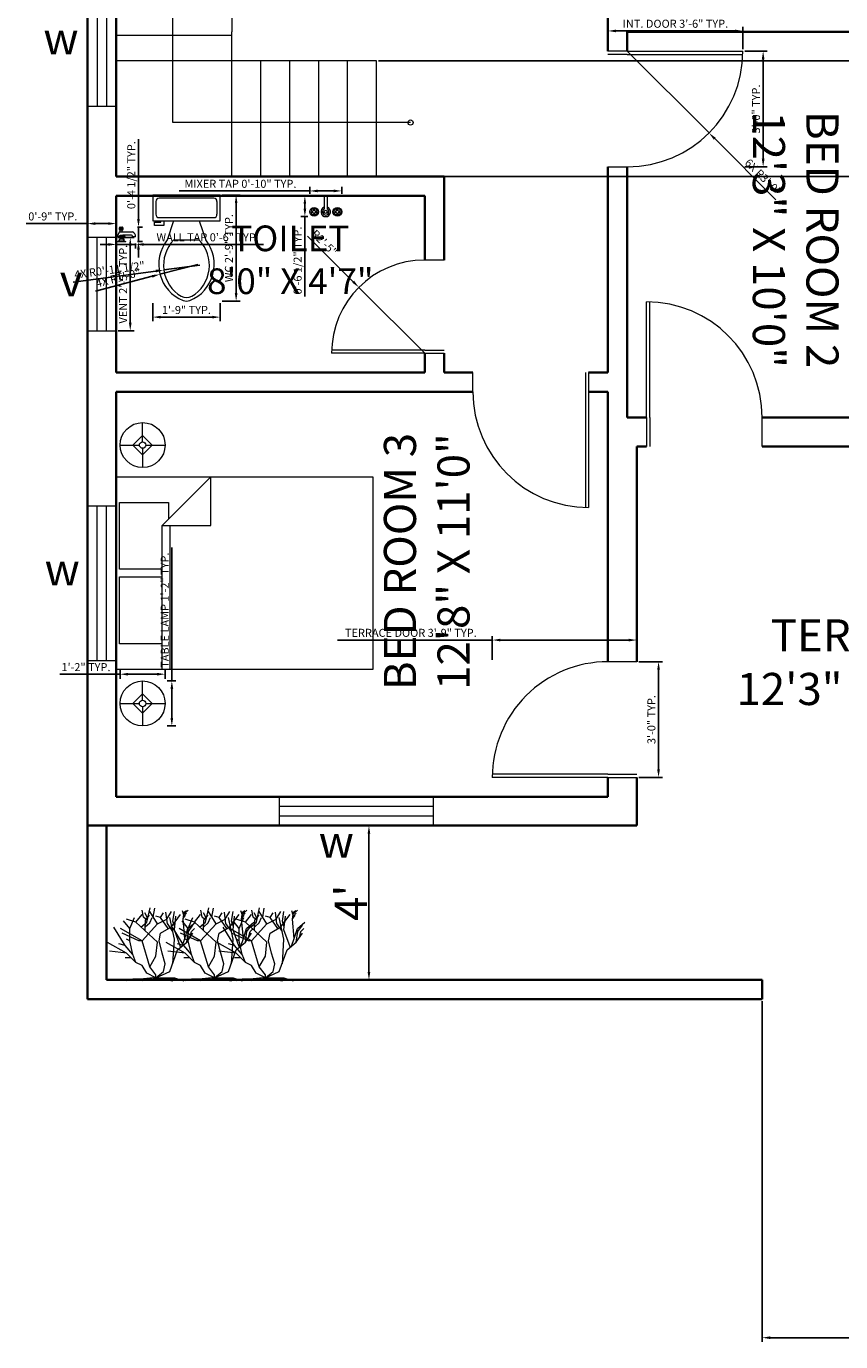
# Model space of a CAD drawing. Units: inches. Extents: x 2729 to 3178, y 5006 to 5809.
# Tile 1 of 4: x 2729 to 2983, y 5006 to 5415. Entities that reach past the tile are written whole.
import ezdxf

# ---------------------------------------------------------------- set-up
doc = ezdxf.new("R2010")
doc.units = ezdxf.units.IN
doc.layers.get('Defpoints').update_dxf_attribs({"color": 72})
for name, color, linetype, lineweight in [('A-ANNO-DIMS', 2, 'Continuous', 18), ('A-ANNO-TEXT', 7, 'Continuous', 18), ('A-AREA-IDEN', 7, 'Continuous', 25), ('A-DOOR', 4, 'Continuous', 18), ('A-FLOR-FIXT', 9, 'Continuous', 18), ('A-FLOR-STRS', 7, 'Continuous', 18), ('A-FURN', 8, 'Continuous', 18), ('A-GLAZ', 4, 'Continuous', 18), ('A-WALL', 7, 'Continuous', 35), ('L-PLNT', 72, 'Continuous', 13)]:
    doc.layers.add(name, color=color, linetype=linetype, lineweight=lineweight)
doc.styles.get("Standard").update_dxf_attribs({"font": 'arial.ttf'})
doc.dimstyles.new('ISO-25', dxfattribs={"dimtxt": 2.5, "dimasz": 2.5, "dimexe": 1.25, "dimexo": 0.625, "dimtad": 1, "dimdec": 0, "dimlunit": 3, "dimtxsty": 'Standard', "dimcen": 2.5, "dimadec": 0, "dimazin": 0, "dimtfac": 1, "dimtdec": 0, "dimtmove": 0, "dimatfit": 3, "dimfxl": 1, "dimarcsym": 0})

# ---------------------------------------------------------------- blocks, each defined once
blk = doc.blocks.new('Toilet - top')
for p, q in [((9.5, -6), (9.5, -2)), ((-8, -8.5), (-8, -8)), ((-7, -8), (-7, -9.5)), ((-4, -8), (-6, -14)), ((4, -8), (6, -14)), ((-10, -8.5), (-8, -8.5)), ((-10, -9.5), (-10, -8.5)), ((-7, -9.5), (-10, -9.5)), ((4, -14), (-4, -14))]:
    blk.add_line(p, q)
blk.add_lwpolyline([(10.5, -8), (10.5, 0), (-10.5, 0), (-10.5, -8)], close=True)
for points in [[(-9.5, -2), (-9.5, -6)], [(8.5, -1), (-8.5, -1)], [(-8.5, -7), (8.5, -7)]]:
    blk.add_lwpolyline(points)
for centre, radius, start, end in [((-8.62, -1.88), 0.884, 81.8699, 188.1301), ((8.62, -1.88), 0.884, 351.8699, 98.1301), ((-8.62, -6.12), 0.884, 171.8699, 278.1301), ((8.62, -6.12), 0.884, 261.8699, 8.1301), ((3.52, -21.58), 12.17, 141.4691, 247.9714), ((4.2, -21.82), 11.33, 136.3677, 238.9468), ((-3.52, -21.58), 12.17, 292.0284, 38.5307), ((-4.2, -21.82), 11.33, 301.053, 43.6321), ((0, -27.88), 4, 245.7318, 294.2682), ((0, -29), 4, 254.8605, 285.1395)]:
    blk.add_arc(centre, radius, start, end)
blk = doc.blocks.new('Bed - Queen')
for p, q in [((0, -80.00003), (0, 0)), ((0, 0), (59.99999, 0)), ((59.99999, 0), (59.99999, -80.00003)), ((7.99999, -1.2), (28.79998, -1.2)), ((7.99999, -14.4), (7.99999, -1.2)), ((28.79998, -1.2), (28.79998, -14.4)), ((31.19999, -1.2), (51.99999, -1.2)), ((31.19999, -14.4), (31.19999, -1.2)), ((51.99999, -1.2), (51.99999, -16.4)), ((0, -14.4), (44.8, -14.4)), ((59.99999, -29.6), (44.8, -14.4)), ((44.8, -14.4), (44.8, -29.6)), ((44.8, -16.8), (0, -16.8)), ((51.99999, -16.4), (46.79936, -16.4)), ((44.8, -29.6), (59.99999, -29.6)), ((59.99999, -80.00003), (0, -80.00003))]:
    blk.add_line(p, q)
blk = doc.blocks.new('Lamp - Table')
for p, q in [((0, 7), (0, 1)), ((-1, 0), (-7, 0)), ((0, 3), (-3, 0)), ((-3, 0), (0, -3)), ((3, 0), (0, 3)), ((0, -3), (3, 0)), ((1, 0), (7, 0)), ((0, -1), (0, -7))]:
    blk.add_line(p, q)
for radius in [7, 1]:
    blk.add_circle((0, 0), radius)
blk = doc.blocks.new('Faucet - Bathroom top')
for p, q in [((-4.107, 0.125), (-4.375, 0.125)), ((-3.75, 0.4788), (-3.75, 0.75)), ((-3.5, 0.482), (-3.5, 0.75)), ((-3.1461, 0.125), (-2.875, 0.125)), ((3.143, 0.125), (2.875, 0.125)), ((3.5, 0.4788), (3.5, 0.75)), ((3.75, 0.482), (3.75, 0.75)), ((4.1039, 0.125), (4.375, 0.125)), ((-4.1039, -0.125), (-4.375, -0.125)), ((-3.75, -0.4821), (-3.75, -0.75)), ((-3.5, -0.4789), (-3.5, -0.75)), ((-3.143, -0.125), (-2.875, -0.125)), ((-0.5, -0.8639), (-0.5, -4.5)), ((0.5, -4.5), (0.5, -0.8631)), ((3.1461, -0.125), (2.875, -0.125)), ((3.5, -0.4821), (3.5, -0.75)), ((3.75, -0.4789), (3.75, -0.75)), ((4.107, -0.125), (4.375, -0.125))]:
    blk.add_line(p, q)
for centre, radius in [((-3.625, 0), 1.375), ((-4.625, 0), 0.2795), ((-3.625, 0), 0.5), ((-3.625, 1), 0.2795), ((-2.625, 0), 0.2795), ((0, 0), 0.5), ((3.625, 0), 1.375), ((2.625, 0), 0.2795), ((3.625, 0), 0.5), ((3.625, 1), 0.2795), ((4.625, 0), 0.2795), ((-3.625, -1), 0.2795), ((3.625, -1), 0.2795)]:
    blk.add_circle(centre, radius)
for centre, radius, start, end in [((-3.625, 0), 1, 105.2407, 164.2093), ((-3.625, 0), 1, 16.44125, 74.07887), ((0, 0), 1.5, 289.6514, 250.3603), ((0, 0), 1, 300.3431, 239.7554), ((3.625, 0), 1, 106.12, 164.0884), ((3.625, 0), 1, 16.23422, 73.90469), ((-3.625, 0), 1, 196.2342, 253.9047), ((-3.625, 0), 1, 286.12, 344.0884), ((3.625, 0), 1, 196.4413, 254.0789), ((3.625, 0), 1, 285.2407, 344.2093), ((0, -4.5), 0.5, 180, 0)]:
    blk.add_arc(centre, radius, start, end)
blk = doc.blocks.new('Faucet - Bathroom side')
for p, q in [((-0.625, 4.25), (0.375, 4.25)), ((-1.625, 0), (-1.375, 0)), ((-1.375, 0), (1.375, 0)), ((-0.88366, 0.25), (0.88424, 0.25)), ((0.375, 3.75), (-0.625, 3.75)), ((-0.625, 3), (3.375, 3)), ((-0.375, 1.625), (-0.625, 1.625)), ((-0.375, 1.375), (-0.625, 1.375)), ((0.48078, 0.75), (-0.47286, 0.75)), ((-0.375, 3), (-0.375, 3.5)), ((0.125, 3.5), (0.125, 3)), ((2.875, 2), (0.375, 2)), ((0.375, 1.625), (0.625, 1.625)), ((0.375, 1.375), (0.625, 1.375)), ((4.375, 1.5), (3.375, 1.5))]:
    blk.add_line(p, q)
for points in [[(-0.625, 3.75), (-0.625, 4.25)], [(-0.375, 4.5), (0.125, 4.5)], [(0.375, 4.25), (0.375, 3.75)], [(0.125, 3.5), (-0.375, 3.5)]]:
    blk.add_lwpolyline(points)
blk.add_lwpolyline([(-0.375, 1), (-0.375, 2), (0.375, 2), (0.375, 1)], close=True)
for centre in [(-0.875, 1.5), (0, 1.5), (0.875, 1.5)]:
    blk.add_circle(centre, 0.27951)
for centre, radius, start, end in [((-0.38253, 4.2575), 0.24259, 88.22243, 181.7776), ((0.13252, 4.2575), 0.24259, 358.2224, 91.77757), ((3.45929, -0.0281), 5.08436, 143.4467, 179.6834), ((-1.75, 1.375), 1.42522, 285.2551, 344.7449), ((-0.38253, 3.7424), 0.24259, 178.2224, 271.7776), ((0.13252, 3.7424), 0.24259, 268.2224, 1.777565), ((1.75, 1.375), 1.42522, 195.2551, 254.7449), ((-2.49562, -0.286), 3.38273, 9.709485, 29.48735), ((2.96867, 1.5936), 0.41699, 347.0192, 102.9808), ((2.70708, 1.4714), 1.66816, 0.9827695, 66.39737)]:
    blk.add_arc(centre, radius, start, end)
blk = doc.blocks.new('*U13')
for p, q in [((-377.952, 463.296), (-329.184, 524.256)), ((-316.7634, 502.285), (-327.6092, 559.9176)), ((-286.512, 498.3226), (-307.4416, 538.0736)), ((-290.3982, 464.5406), (-265.6078, 577.8246)), ((-207.264, 451.104), (-268.224, 548.64)), ((-240.792, 502.285), (-228.3968, 573.8368)), ((-182.88, 499.872), (-158.496, 536.448)), ((-129.1844, 450.6214), (-140.0302, 542.036)), ((-134.112, 487.68), (-97.536, 548.64)), ((-97.536, 426.72), (-24.384, 524.256)), ((-85.7758, 472.4908), (-73.3552, 548.005)), ((-12.9032, 555.9552), (-2.0574, 522.1732)), ((-5.1562, 486.3846), (2.5908, 542.036)), ((-0.508, 508.254), (22.7584, 536.067)), ((1.0414, 526.1356), (35.1536, 559.9176)), ((2.5908, 542.036), (21.209, 555.9552)), ((-463.296, 280.416), (-552.577, 423.037)), ((-426.72, 414.528), (-475.488, 475.488)), ((-377.952, 463.296), (-451.104, 487.68)), ((-426.72, 414.528), (-390.144, 499.872)), ((-207.264, 304.8), (-377.952, 463.296)), ((-338.455, 424.7896), (-290.3982, 464.5406)), ((-329.184, 316.992), (-207.264, 451.104)), ((-296.5958, 484.4034), (-316.7634, 502.285)), ((-305.8922, 396.9512), (-302.7934, 478.4344)), ((-304.3428, 426.7708), (-268.7066, 458.5716)), ((-302.7934, 478.4344), (-270.256, 518.1854)), ((-268.7066, 458.5716), (-250.0884, 500.3038)), ((-182.88, 499.872), (-219.456, 512.064)), ((-207.264, 451.104), (-134.112, 487.68)), ((-121.92, 414.528), (-182.88, 499.872)), ((-182.88, 377.952), (-97.536, 426.72)), ((-85.7758, 389.001), (-129.1844, 452.6026)), ((-73.152, 329.184), (-109.728, 499.872)), ((-70.2564, 426.7708), (-85.7758, 472.4908)), ((-73.152, 402.336), (-60.96, 512.064)), ((8.7884, 335.3562), (-5.1562, 486.3846)), ((-3.6068, 492.3536), (14.986, 518.1854)), ((33.6042, 412.8516), (92.5068, 464.5406)), ((36.576, 390.144), (73.152, 438.912)), ((-329.184, 316.992), (-499.872, 414.528)), ((-353.568, 316.992), (-487.68, 377.952)), ((-426.72, 316.992), (-451.104, 329.184)), ((-426.72, 316.992), (-426.72, 414.528)), ((-402.336, 207.264), (-426.72, 316.992)), ((-329.184, 316.992), (-353.568, 316.992)), ((-268.224, 109.728), (-329.184, 316.992)), ((-195.072, 316.992), (-182.88, 377.952)), ((-170.688, 219.456), (-195.072, 316.992)), ((-85.344, 134.112), (-73.152, 329.184)), ((-24.384, 268.224), (-73.152, 402.336)), ((-12.192, 274.32), (8.7884, 335.3562)), ((8.7884, 335.3562), (33.6042, 412.8516)), ((24.384, 304.8), (36.576, 390.144)), ((24.384, 304.8), (73.152, 377.952)), ((48.768, 341.376), (60.96, 390.144)), ((60.96, 390.144), (85.344, 414.528)), ((-451.104, 219.456), (-601.0402, 303.8094)), ((-451.104, 219.456), (-587.4512, 234.2388)), ((-463.296, 280.416), (-512.064, 292.608)), ((-402.336, 207.264), (-463.296, 280.416)), ((-377.952, 146.304), (-451.104, 219.456)), ((-219.456, 195.072), (-207.264, 304.8)), ((-146.304, 134.112), (-170.688, 219.456)), ((-109.728, 73.152), (-48.768, 243.84)), ((-48.768, 243.84), (24.384, 304.8)), ((-414.528, 182.88), (-463.296, 182.88)), ((-377.952, 146.304), (-402.336, 207.264)), ((-329.184, 121.92), (-377.952, 146.304)), ((-292.608, 60.96), (-329.184, 121.92)), ((-268.224, 109.728), (-219.456, 195.072)), ((-219.456, 48.768), (-268.224, 109.728)), ((-158.496, 73.152), (-146.304, 134.112)), ((-402.336, 12.192), (-451.104, 0)), ((-341.376, 12.192), (-402.336, 12.192)), ((-243.84, 24.384), (-341.376, 12.192)), ((-243.84, 24.384), (-329.184, 0)), ((-219.456, 24.384), (-292.608, 60.96)), ((-243.84, 24.384), (-195.072, 24.384)), ((-219.456, 24.384), (-109.728, 73.152)), ((-219.456, 24.384), (-158.496, 73.152)), ((-219.456, 24.384), (-219.456, 48.768)), ((-219.456, 24.384), (-73.152, 24.384)), ((-195.072, 24.384), (-158.496, 12.192)), ((-158.496, 12.192), (-85.344, 0)), ((-73.152, 24.384), (0, 0))]:
    blk.add_line(p, q)
blk = doc.blocks.new('*D17')
at = {"layer": 'A-ANNO-DIMS', "color": 0, "lineweight": -2, "transparency": 16777216}
for p, q in [((2754.8, 5166.64), (2837.06, 5166.64)), ((2835.81, 5164.14), (2835.81, 5121.14)), ((2754.8, 5118.64), (2837.06, 5118.64))]:
    blk.add_line(p, q, dxfattribs=at)
at = {"layer": 'A-ANNO-DIMS', "color": 0, "transparency": 16777216}
for points in [[(2835.39, 5164.14), (2836.23, 5164.14), (2835.81, 5166.64)], [(2835.39, 5121.14), (2836.23, 5121.14), (2835.81, 5118.64)]]:
    blk.add_solid(points, dxfattribs=at)
at = {"layer": 'Defpoints', "color": 0, "transparency": 16777216}
for p in [(2754.18, 5166.64), (2754.18, 5118.64), (2835.81, 5118.64)]:
    blk.add_point(p, dxfattribs=at)
at = {"layer": 'A-ANNO-DIMS', "color": 0, "transparency": 16777216, "insert": (2830.19, 5142.64), "char_height": 2.5, "attachment_point": 5, "rotation": 90}
blk.add_mtext("{\\H4x;4'}", dxfattribs=at)
blk = doc.blocks.new('WIN-48IN')
for p, q in [((48, 9), (0, 9)), ((0, 9), (0, 0)), ((48, 0), (48, 9)), ((48, 6), (0, 6)), ((0, 3), (48, 3)), ((0, 0), (48, 0))]:
    blk.add_line(p, q)
blk = doc.blocks.new('DOOR-36IN-JAMB6')
for p, q in [((0, 6), (0, 42)), ((1, 6), (1, 42)), ((0, 6), (0, 0)), ((1, 6), (1, 0)), ((36, 0), (36, 6))]:
    blk.add_line(p, q)
blk.add_arc((0, 6), 36, 0, 90)
blk = doc.blocks.new('VENT-29IN')
for p, q in [((29, 9), (0, 9)), ((0, 9), (0, 0)), ((29, 0), (29, 9)), ((29, 6), (0, 6)), ((0, 3), (29, 3)), ((0, 0), (29, 0))]:
    blk.add_line(p, q)
blk = doc.blocks.new('DOOR-36IN-JAMB9')
for p, q in [((0, 9), (0, 45)), ((1, 9), (1, 45)), ((0, 9), (0, 0)), ((1, 9), (1, 0)), ((36, 0), (36, 9))]:
    blk.add_line(p, q)
blk.add_arc((0, 9), 36, 0, 90)
blk = doc.blocks.new('*D29')
at = {"layer": 'A-ANNO-DIMS', "color": 0, "lineweight": -2, "transparency": 16777216}
for p, q in [((2774.48, 5211.66), (2774.48, 5253.23)), ((2773, 5211.66), (2775.73, 5211.66)), ((2774.48, 5200.16), (2774.48, 5209.16)), ((2773, 5197.66), (2775.73, 5197.66))]:
    blk.add_line(p, q, dxfattribs=at)
at = {"layer": 'A-ANNO-DIMS', "color": 0, "transparency": 16777216}
for points in [[(2774.06, 5209.16), (2774.9, 5209.16), (2774.48, 5211.66)], [(2774.06, 5200.16), (2774.9, 5200.16), (2774.48, 5197.66)]]:
    blk.add_solid(points, dxfattribs=at)
at = {"layer": 'Defpoints', "color": 0, "transparency": 16777216}
for p in [(2772.38, 5211.66), (2774.48, 5211.66), (2772.38, 5197.66)]:
    blk.add_point(p, dxfattribs=at)
at = {"layer": 'A-ANNO-DIMS', "color": 0, "transparency": 16777216, "insert": (2772.6, 5233.69), "char_height": 2.5, "attachment_point": 5, "rotation": 90}
blk.add_mtext('TABLE LAMP 1\'-2" TYP.', dxfattribs=at)
blk = doc.blocks.new('*D30')
at = {"layer": 'A-ANNO-DIMS', "color": 0, "lineweight": -2, "transparency": 16777216}
for p, q in [((2758.38, 5212.29), (2758.38, 5215.01)), ((2772.38, 5212.29), (2772.38, 5215.01)), ((2758.38, 5213.76), (2739.62, 5213.76)), ((2769.88, 5213.76), (2760.88, 5213.76))]:
    blk.add_line(p, q, dxfattribs=at)
at = {"layer": 'A-ANNO-DIMS', "color": 0, "transparency": 16777216}
for points in [[(2760.88, 5214.18), (2760.88, 5213.34), (2758.38, 5213.76)], [(2769.88, 5214.18), (2769.88, 5213.34), (2772.38, 5213.76)]]:
    blk.add_solid(points, dxfattribs=at)
at = {"layer": 'Defpoints', "color": 0, "transparency": 16777216}
for p in [(2758.38, 5213.76), (2758.38, 5211.66), (2772.38, 5211.66)]:
    blk.add_point(p, dxfattribs=at)
at = {"layer": 'A-ANNO-DIMS', "color": 0, "transparency": 16777216, "insert": (2747.75, 5215.64), "char_height": 2.5, "attachment_point": 5}
blk.add_mtext('1\'-2" TYP.', dxfattribs=at)
blk = doc.blocks.new('*D33')
at = {"layer": 'A-ANNO-DIMS', "color": 0, "lineweight": -2, "transparency": 16777216}
for p, q in [((2754.7, 5347.5), (2752.2, 5347.5)), ((2757.2, 5347.78), (2757.2, 5346.25)), ((2757.2, 5347.5), (2763.2, 5347.5)), ((2763.2, 5347.78), (2763.2, 5346.25)), ((2765.7, 5347.5), (2803.03, 5347.5))]:
    blk.add_line(p, q, dxfattribs=at)
at = {"layer": 'A-ANNO-DIMS', "color": 0, "transparency": 16777216}
for points in [[(2754.7, 5347.92), (2754.7, 5347.08), (2757.2, 5347.5)], [(2765.7, 5347.92), (2765.7, 5347.08), (2763.2, 5347.5)]]:
    blk.add_solid(points, dxfattribs=at)
at = {"layer": 'Defpoints', "color": 0, "transparency": 16777216}
for p in [(2757.2, 5348.4), (2763.2, 5348.4), (2763.2, 5347.5)]:
    blk.add_point(p, dxfattribs=at)
at = {"layer": 'A-ANNO-DIMS', "color": 0, "transparency": 16777216, "insert": (2785.61, 5349.4), "char_height": 2.5, "attachment_point": 5}
blk.add_mtext('WALL TAP 0\'-6" TYP.', dxfattribs=at)
blk = doc.blocks.new('*D34')
at = {"layer": 'A-ANNO-DIMS', "color": 0, "lineweight": -2, "transparency": 16777216}
for p, q in [((2764.1, 5355.4), (2764.1, 5380.22)), ((2763.82, 5352.9), (2765.35, 5352.9)), ((2764.1, 5348.4), (2764.1, 5352.9)), ((2763.82, 5348.4), (2765.35, 5348.4)), ((2764.1, 5345.9), (2764.1, 5343.4))]:
    blk.add_line(p, q, dxfattribs=at)
at = {"layer": 'A-ANNO-DIMS', "color": 0, "transparency": 16777216}
for points in [[(2763.68, 5355.4), (2764.51, 5355.4), (2764.1, 5352.9)], [(2763.68, 5345.9), (2764.51, 5345.9), (2764.1, 5348.4)]]:
    blk.add_solid(points, dxfattribs=at)
at = {"layer": 'Defpoints', "color": 0, "transparency": 16777216}
for p in [(2763.2, 5352.9), (2764.1, 5352.9), (2763.2, 5348.4)]:
    blk.add_point(p, dxfattribs=at)
at = {"layer": 'A-ANNO-DIMS', "color": 0, "transparency": 16777216, "insert": (2762.18, 5369.06), "char_height": 2.5, "attachment_point": 5, "rotation": 90}
blk.add_mtext('0\'-4 1/2" TYP.', dxfattribs=at)
blk = doc.blocks.new('*D35')
at = {"layer": 'A-ANNO-DIMS', "color": 0, "lineweight": -2, "transparency": 16777216}
for p, q in [((2910.18, 5408.26), (2910.18, 5415.19)), ((2912.68, 5413.94), (2949.68, 5413.94)), ((2952.18, 5408.26), (2952.18, 5415.19))]:
    blk.add_line(p, q, dxfattribs=at)
at = {"layer": 'A-ANNO-DIMS', "color": 0, "transparency": 16777216}
for points in [[(2912.68, 5414.35), (2912.68, 5413.52), (2910.18, 5413.94)], [(2949.68, 5414.35), (2949.68, 5413.52), (2952.18, 5413.94)]]:
    blk.add_solid(points, dxfattribs=at)
at = {"layer": 'Defpoints', "color": 0, "transparency": 16777216}
for p in [(2952.18, 5413.94), (2910.18, 5407.64), (2952.18, 5407.64)]:
    blk.add_point(p, dxfattribs=at)
at = {"layer": 'A-ANNO-DIMS', "color": 0, "transparency": 16777216, "insert": (2931.18, 5415.86), "char_height": 2.5, "attachment_point": 5}
blk.add_mtext('INT. DOOR 3\'-6" TYP.', dxfattribs=at)
blk = doc.blocks.new('*D36')
at = {"layer": 'A-ANNO-DIMS', "color": 0, "lineweight": -2, "transparency": 16777216}
for p, q in [((2952.8, 5407.64), (2959.73, 5407.64)), ((2958.48, 5405.14), (2958.48, 5374.14)), ((2952.8, 5371.64), (2959.73, 5371.64))]:
    blk.add_line(p, q, dxfattribs=at)
at = {"layer": 'A-ANNO-DIMS', "color": 0, "transparency": 16777216}
for points in [[(2958.06, 5405.14), (2958.9, 5405.14), (2958.48, 5407.64)], [(2958.06, 5374.14), (2958.9, 5374.14), (2958.48, 5371.64)]]:
    blk.add_solid(points, dxfattribs=at)
at = {"layer": 'Defpoints', "color": 0, "transparency": 16777216}
for p in [(2952.18, 5407.64), (2952.18, 5371.64), (2958.48, 5371.64)]:
    blk.add_point(p, dxfattribs=at)
at = {"layer": 'A-ANNO-DIMS', "color": 0, "transparency": 16777216, "insert": (2956.58, 5389.64), "char_height": 2.5, "attachment_point": 5, "rotation": 90}
blk.add_mtext('3\'-0" TYP.', dxfattribs=at)
blk = doc.blocks.new('*D39')
at = {"layer": 'A-ANNO-DIMS', "color": 0, "lineweight": -2, "transparency": 16777216}
for p, q in [((2790.15, 5362.88), (2795.73, 5362.88)), ((2794.48, 5332.34), (2794.48, 5360.38)), ((2790.15, 5329.84), (2795.73, 5329.84))]:
    blk.add_line(p, q, dxfattribs=at)
at = {"layer": 'A-ANNO-DIMS', "color": 0, "transparency": 16777216}
for points in [[(2794.07, 5360.38), (2794.9, 5360.38), (2794.48, 5362.88)], [(2794.07, 5332.34), (2794.9, 5332.34), (2794.48, 5329.84)]]:
    blk.add_solid(points, dxfattribs=at)
at = {"layer": 'Defpoints', "color": 0, "transparency": 16777216}
for p in [(2789.53, 5362.88), (2794.48, 5362.88), (2789.53, 5329.84)]:
    blk.add_point(p, dxfattribs=at)
at = {"layer": 'A-ANNO-DIMS', "color": 0, "transparency": 16777216, "insert": (2792.57, 5346.36), "char_height": 2.5, "attachment_point": 5, "rotation": 90}
blk.add_mtext('WC 2\'-9" TYP.', dxfattribs=at)
blk = doc.blocks.new('*D40')
at = {"layer": 'A-ANNO-DIMS', "color": 0, "lineweight": -2, "transparency": 16777216}
for p, q in [((2768.53, 5329.21), (2768.53, 5323.63)), ((2789.53, 5329.21), (2789.53, 5323.63)), ((2771.03, 5324.88), (2787.03, 5324.88))]:
    blk.add_line(p, q, dxfattribs=at)
at = {"layer": 'A-ANNO-DIMS', "color": 0, "transparency": 16777216}
for points in [[(2771.03, 5325.3), (2771.03, 5324.46), (2768.53, 5324.88)], [(2787.03, 5325.3), (2787.03, 5324.46), (2789.53, 5324.88)]]:
    blk.add_solid(points, dxfattribs=at)
at = {"layer": 'Defpoints', "color": 0, "transparency": 16777216}
for p in [(2768.53, 5329.84), (2789.53, 5329.84), (2789.53, 5324.88)]:
    blk.add_point(p, dxfattribs=at)
at = {"layer": 'A-ANNO-DIMS', "color": 0, "transparency": 16777216, "insert": (2779.03, 5326.78), "char_height": 2.5, "attachment_point": 5}
blk.add_mtext('1\'-9" TYP.', dxfattribs=at)
blk = doc.blocks.new('*D41')
at = {"layer": 'A-ANNO-DIMS', "color": 0, "lineweight": -2, "transparency": 16777216}
for p, q in [((2817.37, 5364.15), (2776.76, 5364.15)), ((2817.37, 5363.28), (2817.37, 5365.4)), ((2824.87, 5364.15), (2819.87, 5364.15)), ((2827.37, 5363.28), (2827.37, 5365.4))]:
    blk.add_line(p, q, dxfattribs=at)
at = {"layer": 'A-ANNO-DIMS', "color": 0, "transparency": 16777216}
for points in [[(2819.87, 5364.57), (2819.87, 5363.73), (2817.37, 5364.15)], [(2824.87, 5364.57), (2824.87, 5363.73), (2827.37, 5364.15)]]:
    blk.add_solid(points, dxfattribs=at)
at = {"layer": 'Defpoints', "color": 0, "transparency": 16777216}
for p in [(2817.37, 5364.15), (2817.37, 5362.65), (2827.37, 5362.65)]:
    blk.add_point(p, dxfattribs=at)
at = {"layer": 'A-ANNO-DIMS', "color": 0, "transparency": 16777216, "insert": (2795.82, 5366.05), "char_height": 2.5, "attachment_point": 5}
blk.add_mtext('MIXER TAP 0\'-10" TYP.', dxfattribs=at)
blk = doc.blocks.new('*D42')
at = {"layer": 'A-ANNO-DIMS', "color": 0, "lineweight": -2, "transparency": 16777216}
for p, q in [((2816.75, 5362.65), (2814.62, 5362.65)), ((2815.87, 5360.15), (2815.87, 5358.65)), ((2816.75, 5356.15), (2814.62, 5356.15)), ((2815.87, 5356.15), (2815.87, 5331.34))]:
    blk.add_line(p, q, dxfattribs=at)
at = {"layer": 'A-ANNO-DIMS', "color": 0, "transparency": 16777216}
for points in [[(2815.46, 5360.15), (2816.29, 5360.15), (2815.87, 5362.65)], [(2815.46, 5358.65), (2816.29, 5358.65), (2815.87, 5356.15)]]:
    blk.add_solid(points, dxfattribs=at)
at = {"layer": 'Defpoints', "color": 0, "transparency": 16777216}
for p in [(2817.37, 5362.65), (2815.87, 5356.15), (2817.37, 5356.15)]:
    blk.add_point(p, dxfattribs=at)
at = {"layer": 'A-ANNO-DIMS', "color": 0, "transparency": 16777216, "insert": (2813.95, 5342.49), "char_height": 2.5, "attachment_point": 5, "rotation": 90}
blk.add_mtext('0\'-6 1/2" TYP.', dxfattribs=at)
blk = doc.blocks.new('*D45')
at = {"layer": 'A-ANNO-DIMS', "color": 0, "lineweight": -2, "transparency": 16777216}
for p, q in [((2757.8, 5349.64), (2762.78, 5349.64)), ((2761.53, 5323.14), (2761.53, 5347.14)), ((2757.8, 5320.64), (2762.78, 5320.64))]:
    blk.add_line(p, q, dxfattribs=at)
at = {"layer": 'A-ANNO-DIMS', "color": 0, "transparency": 16777216}
for points in [[(2761.11, 5347.14), (2761.95, 5347.14), (2761.53, 5349.64)], [(2761.11, 5323.14), (2761.95, 5323.14), (2761.53, 5320.64)]]:
    blk.add_solid(points, dxfattribs=at)
at = {"layer": 'Defpoints', "color": 0, "transparency": 16777216}
for p in [(2757.18, 5349.64), (2761.53, 5349.64), (2757.18, 5320.64)]:
    blk.add_point(p, dxfattribs=at)
at = {"layer": 'A-ANNO-DIMS', "color": 0, "transparency": 16777216, "insert": (2759.63, 5335.14), "char_height": 2.5, "attachment_point": 5, "rotation": 90}
blk.add_mtext('VENT 2\'-5" TYP.', dxfattribs=at)
blk = doc.blocks.new('*D46')
at = {"layer": 'A-ANNO-DIMS', "color": 0, "lineweight": -2, "transparency": 16777216}
for p, q in [((2748.18, 5350.26), (2748.18, 5355.24)), ((2757.18, 5350.26), (2757.18, 5355.24)), ((2748.18, 5353.99), (2729.19, 5353.99)), ((2754.68, 5353.99), (2750.68, 5353.99))]:
    blk.add_line(p, q, dxfattribs=at)
at = {"layer": 'A-ANNO-DIMS', "color": 0, "transparency": 16777216}
for points in [[(2750.68, 5354.4), (2750.68, 5353.57), (2748.18, 5353.99)], [(2754.68, 5354.4), (2754.68, 5353.57), (2757.18, 5353.99)]]:
    blk.add_solid(points, dxfattribs=at)
at = {"layer": 'Defpoints', "color": 0, "transparency": 16777216}
for p in [(2748.18, 5353.99), (2748.18, 5349.64), (2757.18, 5349.64)]:
    blk.add_point(p, dxfattribs=at)
at = {"layer": 'A-ANNO-DIMS', "color": 0, "transparency": 16777216, "insert": (2737.43, 5355.89), "char_height": 2.5, "attachment_point": 5}
blk.add_mtext('0\'-9" TYP.', dxfattribs=at)
blk = doc.blocks.new('*D47')
at = {"layer": 'A-ANNO-DIMS', "color": 0, "lineweight": -2, "transparency": 16777216}
for p, q in [((2874.18, 5224.39), (2826.02, 5224.39)), ((2874.18, 5218.26), (2874.18, 5225.64)), ((2916.68, 5224.39), (2876.68, 5224.39)), ((2919.18, 5218.26), (2919.18, 5225.64))]:
    blk.add_line(p, q, dxfattribs=at)
at = {"layer": 'A-ANNO-DIMS', "color": 0, "transparency": 16777216}
for points in [[(2876.68, 5224.8), (2876.68, 5223.97), (2874.18, 5224.39)], [(2916.68, 5224.8), (2916.68, 5223.97), (2919.18, 5224.39)]]:
    blk.add_solid(points, dxfattribs=at)
at = {"layer": 'Defpoints', "color": 0, "transparency": 16777216}
for p in [(2874.18, 5224.39), (2874.18, 5217.64), (2919.18, 5217.64)]:
    blk.add_point(p, dxfattribs=at)
at = {"layer": 'A-ANNO-DIMS', "color": 0, "transparency": 16777216, "insert": (2848.85, 5226.31), "char_height": 2.5, "attachment_point": 5}
blk.add_mtext('TERRACE DOOR 3\'-9" TYP.', dxfattribs=at)
blk = doc.blocks.new('*D48')
at = {"layer": 'A-ANNO-DIMS', "color": 0, "lineweight": -2, "transparency": 16777216}
for p, q in [((2919.8, 5217.64), (2927.18, 5217.64)), ((2925.93, 5184.14), (2925.93, 5215.14)), ((2919.8, 5181.64), (2927.18, 5181.64))]:
    blk.add_line(p, q, dxfattribs=at)
at = {"layer": 'A-ANNO-DIMS', "color": 0, "transparency": 16777216}
for points in [[(2925.51, 5215.14), (2926.35, 5215.14), (2925.93, 5217.64)], [(2925.51, 5184.14), (2926.35, 5184.14), (2925.93, 5181.64)]]:
    blk.add_solid(points, dxfattribs=at)
at = {"layer": 'Defpoints', "color": 0, "transparency": 16777216}
for p in [(2919.18, 5217.64), (2925.93, 5217.64), (2919.18, 5181.64)]:
    blk.add_point(p, dxfattribs=at)
at = {"layer": 'A-ANNO-DIMS', "color": 0, "transparency": 16777216, "insert": (2924.03, 5199.64), "char_height": 2.5, "attachment_point": 5, "rotation": 90}
blk.add_mtext('3\'-0" TYP.', dxfattribs=at)
blk = doc.blocks.new('*D51')
at = {"layer": 'A-ANNO-DIMS', "color": 0, "lineweight": -2, "transparency": 16777216}
for p, q in [((2958.18, 5112.01), (2958.18, 5006.05)), ((3054.18, 5112.01), (3054.18, 5006.05)), ((2960.68, 5007.3), (3051.68, 5007.3))]:
    blk.add_line(p, q, dxfattribs=at)
at = {"layer": 'A-ANNO-DIMS', "color": 0, "transparency": 16777216}
for points in [[(2960.68, 5007.72), (2960.68, 5006.88), (2958.18, 5007.3)], [(3051.68, 5007.72), (3051.68, 5006.88), (3054.18, 5007.3)]]:
    blk.add_solid(points, dxfattribs=at)
at = {"layer": 'Defpoints', "color": 0, "transparency": 16777216}
for p in [(2958.18, 5112.64), (3054.18, 5112.64), (3054.18, 5007.3)]:
    blk.add_point(p, dxfattribs=at)
at = {"layer": 'A-ANNO-DIMS', "color": 0, "transparency": 16777216, "insert": (3006.18, 5009.2), "char_height": 2.5, "attachment_point": 5}
blk.add_mtext('8\'-0"', dxfattribs=at)
blk = doc.blocks.new('*D53')
at = {"layer": 'A-ANNO-DIMS', "color": 0, "lineweight": -2, "transparency": 16777216}
for p, q in [((2838.8, 5404.64), (3177.73, 5404.64)), ((3176.48, 5371.14), (3176.48, 5402.14)), ((2838.8, 5368.64), (3177.73, 5368.64))]:
    blk.add_line(p, q, dxfattribs=at)
at = {"layer": 'A-ANNO-DIMS', "color": 0, "transparency": 16777216}
for points in [[(3176.06, 5402.14), (3176.9, 5402.14), (3176.48, 5404.64)], [(3176.06, 5371.14), (3176.9, 5371.14), (3176.48, 5368.64)]]:
    blk.add_solid(points, dxfattribs=at)
at = {"layer": 'Defpoints', "color": 0, "transparency": 16777216}
for p in [(2838.18, 5404.64), (3176.48, 5404.64), (2838.18, 5368.64)]:
    blk.add_point(p, dxfattribs=at)
at = {"layer": 'A-ANNO-DIMS', "color": 0, "transparency": 16777216, "insert": (3174.58, 5386.64), "char_height": 2.5, "attachment_point": 5, "rotation": 90}
blk.add_mtext('3\'-0"', dxfattribs=at)
blk = doc.blocks.new('*D54')
at = {"layer": 'A-ANNO-DIMS', "color": 0, "lineweight": -2, "transparency": 16777216}
for p, q in [((2916.18, 5407.64), (2941.64, 5382.18)), ((2962.45, 5361.37), (2943.4, 5380.42))]:
    blk.add_line(p, q, dxfattribs=at)
at = {"layer": 'A-ANNO-DIMS', "color": 0, "transparency": 16777216}
blk.add_solid([(2943.7, 5380.71), (2943.11, 5380.12), (2941.64, 5382.18)], dxfattribs=at)
at = {"layer": 'Defpoints', "color": 0, "transparency": 16777216}
for p in [(2916.18, 5407.64), (2941.64, 5382.18)]:
    blk.add_point(p, dxfattribs=at)
at = {"layer": 'A-ANNO-DIMS', "color": 0, "transparency": 16777216, "insert": (2958.26, 5368.26), "char_height": 2.5, "attachment_point": 5, "rotation": 315.0044}
blk.add_mtext('6X R3\'-0"', dxfattribs=at)
blk = doc.blocks.new('*D55')
at = {"layer": 'A-ANNO-DIMS', "color": 0, "lineweight": -2, "transparency": 16777216}
for p, q in [((2816.73, 5350.08), (2830.91, 5335.91)), ((2853.18, 5313.64), (2832.67, 5334.14))]:
    blk.add_line(p, q, dxfattribs=at)
at = {"layer": 'A-ANNO-DIMS', "color": 0, "transparency": 16777216}
blk.add_solid([(2831.2, 5336.21), (2830.61, 5335.62), (2832.67, 5334.14)], dxfattribs=at)
at = {"layer": 'Defpoints', "color": 0, "transparency": 16777216}
for p in [(2832.67, 5334.14), (2853.18, 5313.64)]:
    blk.add_point(p, dxfattribs=at)
at = {"layer": 'A-ANNO-DIMS', "color": 0, "transparency": 16777216, "insert": (2821.71, 5347.79), "char_height": 2.5, "attachment_point": 5, "rotation": 315.0001}
blk.add_mtext('R2\'-5"', dxfattribs=at)
blk = doc.blocks.new('*D58')
at = {"layer": 'A-ANNO-DIMS', "color": 0, "lineweight": -2, "transparency": 16777216}
for p, q in [((2782.55, 5341.3), (2770.78, 5338.21)), ((2750.7, 5332.94), (2768.36, 5337.58))]:
    blk.add_line(p, q, dxfattribs=at)
at = {"layer": 'A-ANNO-DIMS', "color": 0, "transparency": 16777216}
blk.add_solid([(2768.25, 5337.98), (2768.46, 5337.17), (2770.78, 5338.21)], dxfattribs=at)
at = {"layer": 'Defpoints', "color": 0, "transparency": 16777216}
for p in [(2770.78, 5338.21), (2782.55, 5341.3)]:
    blk.add_point(p, dxfattribs=at)
at = {"layer": 'A-ANNO-DIMS', "color": 0, "transparency": 16777216, "insert": (2757.84, 5336.78), "char_height": 2.5, "attachment_point": 5, "rotation": 14.7189}
blk.add_mtext('4X R1\'-0"', dxfattribs=at)
blk = doc.blocks.new('*D59')
at = {"layer": 'A-ANNO-DIMS', "color": 0, "lineweight": -2, "transparency": 16777216}
for p, q in [((2743.73, 5335.75), (2769.52, 5339.22)), ((2783.23, 5341.07), (2772, 5339.56))]:
    blk.add_line(p, q, dxfattribs=at)
at = {"layer": 'A-ANNO-DIMS', "color": 0, "transparency": 16777216}
blk.add_solid([(2769.47, 5339.64), (2769.58, 5338.81), (2772, 5339.56)], dxfattribs=at)
at = {"layer": 'Defpoints', "color": 0, "transparency": 16777216}
for p in [(2772, 5339.56), (2783.23, 5341.07)]:
    blk.add_point(p, dxfattribs=at)
at = {"layer": 'A-ANNO-DIMS', "color": 0, "transparency": 16777216, "insert": (2755.13, 5339.22), "char_height": 2.5, "attachment_point": 5, "rotation": 7.6592}
blk.add_mtext('4X R0\'-11 1/2"', dxfattribs=at)

msp = doc.modelspace()

# ---------------------------------------------------------------- linework, layer by layer
at = {"layer": 'A-DOOR'}
for p, q in [((2859.18, 5342.64), (2853.18, 5342.64)), ((2853.18, 5314.64), (2824.18, 5314.64)), ((2853.18, 5313.64), (2824.18, 5313.64)), ((2853.18, 5314.64), (2859.18, 5314.64)), ((2853.18, 5313.64), (2859.18, 5313.64)), ((2868.18, 5301.64), (2868.18, 5307.64)), ((2903.18, 5307.64), (2903.18, 5265.64)), ((2904.18, 5307.64), (2904.18, 5301.64)), ((2904.18, 5307.64), (2904.18, 5265.64))]:
    msp.add_line(p, q, dxfattribs=at)
for centre, radius, start, end in [((2853.18, 5313.64), 29, 90, 180), ((2904.18, 5301.64), 36, 180, 270)]:
    msp.add_arc(centre, radius, start, end, dxfattribs=at)
at = {"layer": 'A-FLOR-STRS'}
for p, q in [((2774.75, 5385.44), (2774.75, 5537.18)), ((2793.18, 5419.64), (2793.18, 5413.64)), ((2757.18, 5412.64), (2793.18, 5412.64)), ((2793.18, 5368.64), (2793.18, 5413.64)), ((2838.18, 5404.64), (2757.18, 5404.64)), ((2802.18, 5368.64), (2802.18, 5404.64)), ((2811.18, 5368.64), (2811.18, 5404.64)), ((2820.18, 5368.64), (2820.18, 5404.64)), ((2829.18, 5368.64), (2829.18, 5404.64)), ((2838.18, 5368.64), (2838.18, 5404.64)), ((2848.75, 5385.44), (2774.75, 5385.44))]:
    msp.add_line(p, q, dxfattribs=at)
msp.add_circle((2848.75, 5385.44), 0.805, dxfattribs=at)
at = {"layer": 'A-WALL'}
for p, q in [((2748.18, 5112.64), (2748.18, 5760.64)), ((2757.18, 5419.64), (2757.18, 5413.64)), ((2910.18, 5419.64), (2910.18, 5407.64)), ((2757.18, 5368.64), (2757.18, 5413.64)), ((2916.18, 5413.64), (3063.18, 5413.64)), ((2916.18, 5413.64), (2916.18, 5407.64)), ((2916.18, 5413.64), (2916.18, 5407.64)), ((2910.18, 5371.64), (2910.18, 5307.64)), ((2916.18, 5371.64), (2916.18, 5293.64)), ((2859.18, 5368.64), (2757.18, 5368.64)), ((2859.18, 5362.64), (2859.18, 5368.64)), ((2757.18, 5307.64), (2757.18, 5362.64)), ((2853.18, 5362.64), (2757.18, 5362.64)), ((2853.18, 5342.64), (2853.18, 5362.64)), ((2859.18, 5342.64), (2859.18, 5362.64)), ((2853.18, 5307.64), (2853.18, 5313.64)), ((2853.18, 5307.64), (2853.18, 5313.64)), ((2859.18, 5307.64), (2859.18, 5313.64)), ((2853.18, 5307.64), (2757.18, 5307.64)), ((2868.18, 5307.64), (2859.18, 5307.64)), ((2910.18, 5307.64), (2904.18, 5307.64)), ((2910.18, 5307.64), (2904.18, 5307.64)), ((2859.18, 5301.64), (2757.18, 5301.64)), ((2757.18, 5175.64), (2757.18, 5301.64)), ((2859.18, 5301.64), (2868.18, 5301.64)), ((2910.18, 5301.64), (2904.18, 5301.64)), ((2904.18, 5301.64), (2910.18, 5301.64)), ((2904.18, 5301.64), (2910.18, 5301.64)), ((2910.18, 5301.64), (2910.18, 5217.64)), ((2916.18, 5301.64), (2916.18, 5293.64)), ((2916.18, 5293.64), (2922.18, 5293.64)), ((2916.18, 5293.64), (2922.18, 5293.64)), ((2958.18, 5293.64), (3063.18, 5293.64)), ((2919.18, 5284.64), (2919.18, 5217.64)), ((2919.18, 5284.64), (2922.18, 5284.64)), ((2958.18, 5284.64), (3063.18, 5284.64)), ((2910.18, 5175.64), (2910.18, 5181.64)), ((2910.18, 5181.64), (2910.18, 5175.64)), ((2919.18, 5181.64), (2919.18, 5175.64)), ((2910.18, 5175.64), (2757.18, 5175.64)), ((2919.18, 5175.64), (2919.18, 5166.64)), ((2757.18, 5166.64), (2748.18, 5166.64)), ((2754.18, 5118.64), (2754.18, 5166.64)), ((2757.18, 5166.64), (2754.18, 5166.64)), ((2910.18, 5166.64), (2757.18, 5166.64)), ((2919.18, 5166.64), (2910.18, 5166.64)), ((2958.18, 5118.64), (2754.18, 5118.64)), ((2958.18, 5112.64), (2958.18, 5118.64)), ((2958.18, 5112.64), (2748.18, 5112.64))]:
    msp.add_line(p, q, dxfattribs=at)

# ---------------------------------------------------------------- block references
at = {"layer": 'A-DOOR'}
for name, p, rotation in [('DOOR-36IN-JAMB6', (2910.18, 5407.64), 269.9999999999998), ('DOOR-36IN-JAMB9', (2919.18, 5181.64), 89.99999999999928)]:
    msp.add_blockref(name, p, dxfattribs=dict(at, rotation=rotation))
msp.add_blockref('DOOR-36IN-JAMB9', (2922.18, 5284.64), dxfattribs=at)
at = {"layer": 'A-FLOR-FIXT'}
for name, p in [('Toilet - top', (2779.03, 5362.88)), ('Faucet - Bathroom side', (2758.82, 5348.4))]:
    msp.add_blockref(name, p, dxfattribs=at)
at = {"layer": 'A-FLOR-FIXT', "rotation": 180}
msp.add_blockref('Faucet - Bathroom top', (2822.37, 5357.65), dxfattribs=at)
at = {"layer": 'A-FURN', "rotation": 90}
for name, p in [('Lamp - Table', (2765.38, 5285.07)), ('Bed - Queen', (2757.03, 5215.23)), ('Lamp - Table', (2765.38, 5204.66))]:
    msp.add_blockref(name, p, dxfattribs=at)
at = {"layer": 'A-GLAZ'}
for name, p, rotation in [('WIN-48IN', (2757.26, 5390.54), 89.99999999999935), ('VENT-29IN', (2757.18, 5320.64), 90.00000000000048), ('WIN-48IN', (2757.12, 5218.04), 89.99999999999962)]:
    msp.add_blockref(name, p, dxfattribs=dict(at, rotation=rotation))
msp.add_blockref('WIN-48IN', (2807.9, 5166.64), dxfattribs=at)
at = {"layer": 'L-PLNT', "xscale": 0.0393700787401575, "yscale": 0.0393700787401575, "zscale": 0.0393700787401575}
for p in [(2778.17, 5118.34), (2796.4, 5118.34), (2812.24, 5118.34)]:
    msp.add_blockref('*U13', p, dxfattribs=at)

# ---------------------------------------------------------------- texts
at = {"layer": 'A-ANNO-TEXT', "char_height": 10, "attachment_point": 1}
for s, width, insert in [('w', 11.1436, (2734.5, 5416.61)), ('v', 9.2139, (2739.59, 5341.31)), ('w', 11.1436, (2734.88, 5251.39)), ('w', 11.1436, (2820.18, 5166.64))]:
    msp.add_mtext_dynamic_manual_height_columns(s, width=width, gutter_width=12.5, heights=[0], dxfattribs=dict(at, insert=insert))
at = {"layer": 'A-AREA-IDEN', "char_height": 10, "attachment_point": 1}
for s, insert, rotation in [('\\pxqc,t2;BED ROOM 2\\P12\'3" X 10\'0"', (2981.94, 5396.04), 270), ('\\pxqc,t2;BED ROOM 3\\P12\'8" X 11\'0"', (2840.46, 5201.78), 90)]:
    msp.add_mtext_dynamic_manual_height_columns(s, width=94.0844, gutter_width=12.5, heights=[0], dxfattribs=dict(at, insert=insert, rotation=rotation))
at = {"layer": 'A-AREA-IDEN', "attachment_point": 1}
for s, width, insert, char_height in [('\\pxqc;TOILET\\P8\'0" X 4\'7"', 56.6074, (2783.03, 5353.39), 8), ('\\pxqc;TERRACE\\P12\'3" X 14\'6"', 103.4579, (2938.41, 5230.84), 10)]:
    msp.add_mtext_dynamic_manual_height_columns(s, width=width, gutter_width=12.5, heights=[0], dxfattribs=dict(at, insert=insert, char_height=char_height))

# ---------------------------------------------------------------- dimensions: what is measured, and where the dimension line sits
at = {"layer": 'A-ANNO-DIMS'}
for base, p1, p2, text, picture, middle in [((2952.18, 5413.94), (2910.18, 5407.64), (2952.18, 5407.64), 'INT. DOOR <> TYP.', '*D35', (2931.18, 5415.86)), ((2763.2, 5347.5), (2757.2, 5348.4), (2763.2, 5348.4), 'WALL TAP <> TYP.', '*D33', (2785.61, 5349.4)), ((2789.53, 5324.88), (2768.53, 5329.84), (2789.53, 5329.84), '<> TYP.', '*D40', (2779.03, 5326.78))]:
    dim = msp.add_linear_dim(base=base, p1=p1, p2=p2, text=text, dimstyle='ISO-25', override={"dimdec": 1, "dimlfac": 1, "dimrnd": 0, "dimzin": 1, "dimdsep": 46, "dimlunit": 4, "dimfrac": 2}, dxfattribs=at)
    dim.commit()
    dim.dimension.update_dxf_attribs({"geometry": picture, "text_midpoint": middle})
dim = msp.add_radius_dim(center=(2916.18, 5407.64), mpoint=(2941.64, 5382.18), text='6X <>', dimstyle='ISO-25', override={"dimdec": 1, "dimlfac": 1, "dimrnd": 0, "dimzin": 1, "dimdsep": 46, "dimlunit": 4, "dimfrac": 2}, dxfattribs=at)
dim.commit()
dim.dimension.update_dxf_attribs({"geometry": '*D54', "text_midpoint": (2956.91, 5366.91), "dimtype": 164})
for base, p1, p2, angle, text, override, picture, middle in [((2958.48, 5371.64), (2952.18, 5407.64), (2952.18, 5371.64), 270, '<> TYP.', {"dimdec": 1, "dimlfac": 1, "dimrnd": 0, "dimzin": 1, "dimdsep": 46, "dimlunit": 4, "dimfrac": 2}, '*D36', (2956.58, 5389.64)), ((2764.1, 5352.9), (2763.2, 5348.4), (2763.2, 5352.9), 90, '<> TYP.', {"dimdec": 1, "dimlfac": 1, "dimrnd": 0, "dimzin": 1, "dimdsep": 46, "dimlunit": 4, "dimfrac": 2}, '*D34', (2762.18, 5369.06)), ((2817.37, 5364.15), (2827.37, 5362.65), (2817.37, 5362.65), 180, 'MIXER TAP <> TYP.', {"dimdec": 1, "dimlfac": 1, "dimrnd": 0, "dimzin": 1, "dimdsep": 46, "dimlunit": 4, "dimfrac": 2}, '*D41', (2795.82, 5366.05)), ((2794.48, 5362.88), (2789.53, 5329.84), (2789.53, 5362.88), 90, 'WC <> TYP.', {"dimdec": 1, "dimlfac": 1, "dimrnd": 0, "dimzin": 1, "dimdsep": 46, "dimlunit": 4, "dimfrac": 2}, '*D39', (2792.57, 5346.36)), ((2815.87, 5356.15), (2817.37, 5362.65), (2817.37, 5356.15), 270, '<> TYP.', {"dimdec": 1, "dimlfac": 1, "dimrnd": 0, "dimzin": 1, "dimdsep": 46, "dimlunit": 4, "dimfrac": 2}, '*D42', (2813.95, 5342.49)), ((2748.18, 5353.99), (2757.18, 5349.64), (2748.18, 5349.64), 180, '<> TYP.', {"dimdec": 1, "dimlfac": 1, "dimrnd": 0, "dimzin": 1, "dimdsep": 46, "dimlunit": 4, "dimfrac": 2}, '*D46', (2737.43, 5355.89)), ((2761.53, 5349.64), (2757.18, 5320.64), (2757.18, 5349.64), 90, 'VENT <> TYP.', {"dimdec": 1, "dimlfac": 1, "dimrnd": 0, "dimzin": 1, "dimdsep": 46, "dimlunit": 4, "dimfrac": 2}, '*D45', (2759.63, 5335.14)), ((2774.48, 5211.66), (2772.38, 5197.66), (2772.38, 5211.66), 90, 'TABLE LAMP <> TYP.', {"dimdec": 1, "dimlfac": 1, "dimrnd": 0, "dimzin": 1, "dimdsep": 46, "dimlunit": 4, "dimfrac": 2}, '*D29', (2772.6, 5233.69)), ((2874.18, 5224.39), (2919.18, 5217.64), (2874.18, 5217.64), 180, 'TERRACE DOOR <> TYP.', {"dimdec": 1, "dimlfac": 1, "dimrnd": 0, "dimzin": 1, "dimdsep": 46, "dimlunit": 4, "dimfrac": 2}, '*D47', (2848.85, 5226.31)), ((2758.38, 5213.76), (2772.38, 5211.66), (2758.38, 5211.66), 180, '<> TYP.', {"dimdec": 1, "dimlfac": 1, "dimrnd": 0, "dimzin": 1, "dimdsep": 46, "dimlunit": 4, "dimfrac": 2}, '*D30', (2747.75, 5215.64)), ((2925.93, 5217.64), (2919.18, 5181.64), (2919.18, 5217.64), 90, '<> TYP.', {"dimdec": 1, "dimlfac": 1, "dimrnd": 0, "dimzin": 1, "dimdsep": 46, "dimlunit": 4, "dimfrac": 2}, '*D48', (2924.03, 5199.64)), ((2835.81, 5118.64), (2754.18, 5166.64), (2754.18, 5118.64), 90, "{\\H4x;4'}", {"dimclrd": 0, "dimclre": 0, "dimclrt": 0}, '*D17', (2830.19, 5142.64))]:
    dim = msp.add_linear_dim(base=base, p1=p1, p2=p2, angle=angle, text=text, dimstyle='ISO-25', override=override, dxfattribs=at)
    dim.commit()
    dim.dimension.update_dxf_attribs({"geometry": picture, "text_midpoint": middle})
dim = msp.add_linear_dim(base=(3176.48, 5404.64), p1=(2838.18, 5368.64), p2=(2838.18, 5404.64), angle=90, dimstyle='ISO-25', override={"dimdec": 1, "dimlfac": 1, "dimrnd": 0, "dimzin": 1, "dimdsep": 46, "dimlunit": 4, "dimfrac": 2}, dxfattribs=at)
dim.commit()
dim.dimension.update_dxf_attribs({"geometry": '*D53', "text_midpoint": (3174.58, 5386.64)})
dim = msp.add_radius_dim(center=(2853.18, 5313.64), mpoint=(2832.67, 5334.14), dimstyle='ISO-25', override={"dimdec": 1, "dimlfac": 1, "dimrnd": 0, "dimzin": 1, "dimdsep": 46, "dimlunit": 4, "dimfrac": 2}, dxfattribs=at)
dim.commit()
dim.dimension.update_dxf_attribs({"geometry": '*D55', "text_midpoint": (2820.37, 5346.45), "dimtype": 164})
for center, mpoint, picture, middle in [((2783.23, 5341.07), (2772, 5339.56), '*D59', (2755.13, 5339.22)), ((2782.55, 5341.3), (2770.78, 5338.21), '*D58', (2757.84, 5336.78))]:
    dim = msp.add_radius_dim(center=center, mpoint=mpoint, text='4X <>', dimstyle='ISO-25', override={"dimdec": 1, "dimlfac": 1, "dimrnd": 0, "dimzin": 1, "dimdsep": 46, "dimlunit": 4, "dimfrac": 2}, dxfattribs=at)
    dim.commit()
    dim.dimension.update_dxf_attribs({"geometry": picture, "text_midpoint": middle})
dim = msp.add_linear_dim(base=(3054.18, 5007.3), p1=(2958.18, 5112.64), p2=(3054.18, 5112.64), dimstyle='ISO-25', override={"dimdec": 1, "dimlfac": 1, "dimrnd": 0, "dimzin": 1, "dimdsep": 46, "dimlunit": 4, "dimfrac": 2}, dxfattribs=at)
dim.commit()
dim.dimension.update_dxf_attribs({"geometry": '*D51', "text_midpoint": (3006.18, 5009.2)})

doc.saveas('drawing.dxf')
